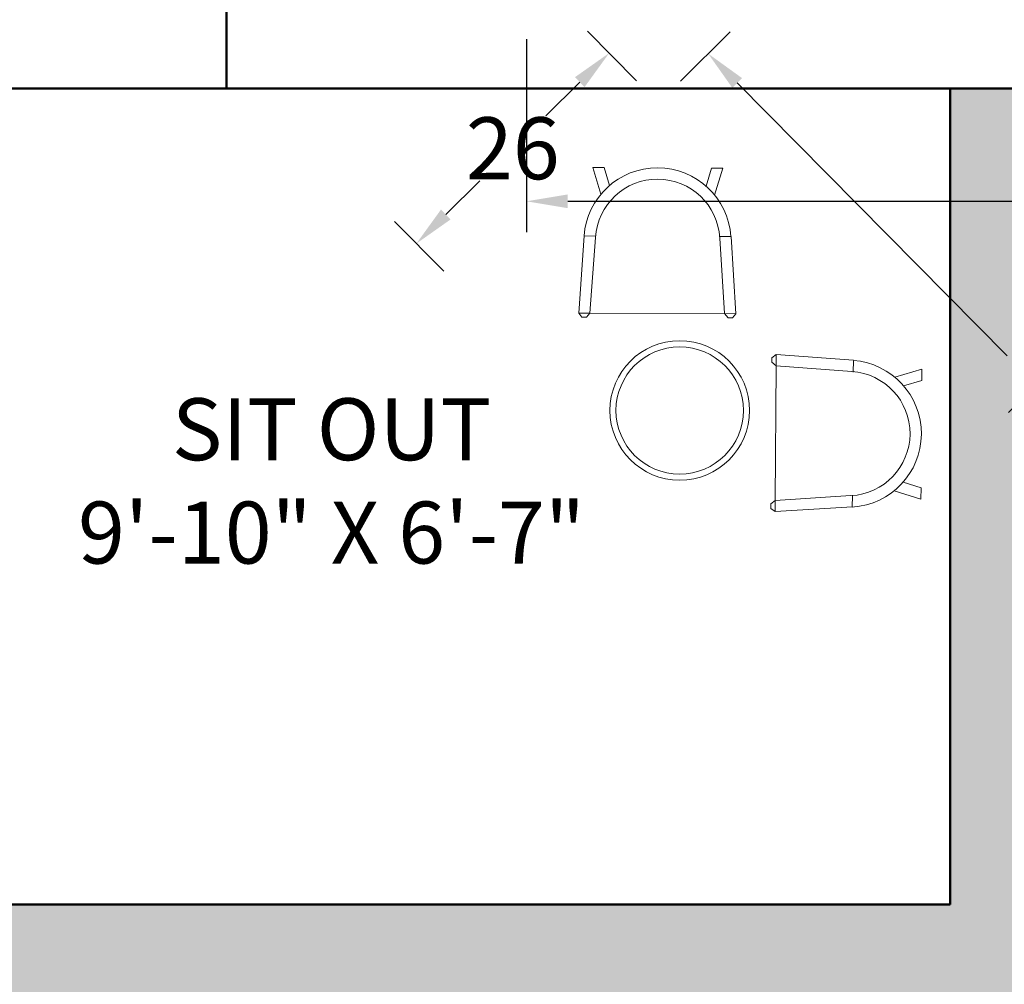
# Model space of a CAD drawing. Units: inches. Extents: x -466983 to 1020, y 324 to 318697.
# Tile 10 of 97: x 641 to 736, y 417 to 511. Entities that reach past the tile are written whole.
import ezdxf

# ---------------------------------------------------------------- set-up
doc = ezdxf.new("R2010")
doc.units = ezdxf.units.IN
doc.header["$MEASUREMENT"] = 0
for name, color, linetype, lineweight in [('A-ANNO-DIMS', 2, 'Continuous', 18), ('A-AREA-IDEN', 7, 'Continuous', 25), ('A-DOOR', 3, 'Continuous', 25), ('A-FLOR-PATT', 252, 'Continuous', 13), ('A-FURN', 8, 'Continuous', 18), ('A-WALL', 7, 'Continuous', 50)]:
    doc.layers.add(name, color=color, linetype=linetype, lineweight=lineweight)
doc.styles.get("Standard").update_dxf_attribs({"font": 'arial.ttf'})
doc.dimstyles.get("Standard").update_dxf_attribs({"dimtxt": 6, "dimasz": 4, "dimexe": 3, "dimexo": 3, "dimgap": 0.09, "dimtad": 0, "dimtih": 1, "dimtoh": 1, "dimdec": 1, "dimzin": 0, "dimdsep": 46, "dimlunit": 3, "dimtxsty": 'Standard', "dimcen": 0.09, "dimadec": 0, "dimazin": 0, "dimtfac": 1, "dimtdec": 1, "dimtofl": 0, "dimtmove": 0, "dimatfit": 3, "dimfxl": 1, "dimtolj": 1, "dimtzin": 0, "dimarcsym": 0})

# ---------------------------------------------------------------- blocks, each defined once
blk = doc.blocks.new('*U41')
for p, q in [((0, 0), (0, -6)), ((40, 0), (40, -6))]:
    blk.add_line(p, q)
blk.add_lwpolyline([(0, 0), (0, 40), (1.75, 40), (1.75, 0)], close=True)
blk.add_arc((0, 0), 40, 0, 90)
blk = doc.blocks.new('Chairs With Tea Table')
for p, q in [((2478.49, 1032.25), (2476.67, 1030.43)), ((2478.49, 1032.25), (2481.53, 1026.6)), ((2542.64, 1032.25), (2539.6, 1026.6)), ((2542.64, 1032.25), (2544.46, 1030.43)), ((2476.67, 1030.43), (2478.7, 1026.65)), ((2544.46, 1030.43), (2542.43, 1026.65)), ((2502.25, 1009.3), (2489.26, 1020.56)), ((2504.05, 1011.1), (2490.83, 1022.62)), ((2517.08, 1011.1), (2530.3, 1022.62)), ((2518.88, 1009.3), (2531.87, 1020.56)), ((2457.66, 1011.37), (2459.48, 1013.2)), ((2459.48, 1013.2), (2463.22, 1011.2)), ((2561.65, 1013.2), (2557.91, 1011.2)), ((2563.47, 1011.37), (2561.65, 1013.2)), ((2457.66, 1011.37), (2463.25, 1008.38)), ((2563.47, 1011.37), (2557.88, 1008.38)), ((2480.67, 987.66), (2502.25, 1009.3)), ((2540.46, 987.66), (2518.88, 1009.3)), ((2469.38, 1000.63), (2480.67, 987.66)), ((2551.75, 1000.63), (2540.46, 987.66)), ((2467.32, 999.05), (2478.9, 985.89)), ((2553.81, 999.05), (2542.23, 985.89))]:
    blk.add_line(p, q)
for points in [[(2488.94, 1020.72), (2490.81, 1022.59, 0.934026), (2467.3, 999.02), (2469.17, 1000.89)], [(2532.19, 1020.72), (2530.32, 1022.59, -0.934026), (2553.83, 999.02), (2551.96, 1000.89)]]:
    blk.add_lwpolyline(points, format="xyb")
for points in [[(2504.05, 1011.1), (2502.25, 1009.3), (2503.49, 1009.16), (2504.22, 1009.9)], [(2517.08, 1011.1), (2518.88, 1009.3), (2517.64, 1009.16), (2516.91, 1009.9)], [(2478.87, 985.86), (2480.67, 987.66), (2480.81, 986.43), (2480.08, 985.69)], [(2542.26, 985.86), (2540.46, 987.66), (2540.32, 986.43), (2541.05, 985.69)]]:
    blk.add_lwpolyline(points, close=True)
for radius in [15.83, 14.45]:
    blk.add_circle((2510.71, 986.6), radius)
for centre, start, end in [((2479.88, 1010.03), 48.307, 221.8389), ((2541.25, 1010.03), 318.1611, 131.693)]:
    blk.add_arc(centre, 14.1, start, end)
blk = doc.blocks.new('*D70')
at = {"layer": 'A-ANNO-DIMS', "color": 0, "lineweight": -2, "transparency": 16777216}
for p, q in [((689.806, 508.686), (689.806, 490.005)), ((810.968, 508.686), (810.968, 490.005)), ((693.806, 493.005), (744.53, 493.005)), ((806.968, 493.005), (756.244, 493.005))]:
    blk.add_line(p, q, dxfattribs=at)
at = {"layer": 'A-ANNO-DIMS', "color": 0, "transparency": 16777216}
for points in [[(693.806, 493.671), (693.806, 492.338), (689.806, 493.005)], [(806.968, 493.671), (806.968, 492.338), (810.968, 493.005)]]:
    blk.add_solid(points, dxfattribs=at)
at = {"layer": 'Defpoints', "color": 0, "transparency": 16777216}
for p in [(689.806, 511.686), (810.968, 511.686), (810.968, 493.005)]:
    blk.add_point(p, dxfattribs=at)
at = {"layer": 'A-ANNO-DIMS', "color": 0, "transparency": 16777216, "insert": (750.387, 493.005), "char_height": 6, "attachment_point": 5}
blk.add_mtext('\\A1;121', dxfattribs=at)
blk = doc.blocks.new('*D113')
at = {"layer": 'A-ANNO-DIMS', "color": 0, "lineweight": -2, "transparency": 16777216}
for p, q in [((704.71, 504.652), (709.525, 509.413)), ((710.204, 504.46), (736.319, 478.049)), ((736.45, 472.553), (741.265, 477.314)), ((739.132, 475.204), (741.944, 472.36)), ((741.944, 472.36), (745.944, 472.36))]:
    blk.add_line(p, q, dxfattribs=at)
at = {"layer": 'A-ANNO-DIMS', "color": 0, "transparency": 16777216}
for points in [[(710.678, 504.928), (709.73, 503.991), (707.392, 507.304)], [(736.794, 478.517), (735.845, 477.58), (739.132, 475.204)]]:
    blk.add_solid(points, dxfattribs=at)
at = {"layer": 'Defpoints', "color": 0, "transparency": 16777216}
for p in [(702.577, 502.543), (739.132, 475.204), (734.317, 470.443)]:
    blk.add_point(p, dxfattribs=at)
at = {"layer": 'A-ANNO-DIMS', "color": 0, "transparency": 16777216, "insert": (783.502, 472.36), "char_height": 6, "attachment_point": 5}
blk.add_mtext('\\A1;TEA TABLE SET 45', dxfattribs=at)
blk = doc.blocks.new('*D114')
at = {"layer": 'A-ANNO-DIMS', "color": 0, "lineweight": -2, "transparency": 16777216}
for p, q in [((700.467, 504.676), (695.706, 509.491)), ((694.971, 504.545), (691.68, 501.29)), ((682.01, 491.729), (685.301, 494.984)), ((681.817, 486.234), (677.056, 491.049))]:
    blk.add_line(p, q, dxfattribs=at)
at = {"layer": 'A-ANNO-DIMS', "color": 0, "transparency": 16777216}
for points in [[(694.503, 505.019), (695.44, 504.071), (697.816, 507.358)], [(681.541, 492.203), (682.478, 491.255), (679.165, 488.916)]]:
    blk.add_solid(points, dxfattribs=at)
at = {"layer": 'Defpoints', "color": 0, "transparency": 16777216}
for p in [(697.816, 507.358), (702.577, 502.543), (683.926, 484.101)]:
    blk.add_point(p, dxfattribs=at)
at = {"layer": 'A-ANNO-DIMS', "color": 0, "transparency": 16777216, "insert": (688.49, 498.137), "char_height": 6, "attachment_point": 5}
blk.add_mtext('\\A1;26', dxfattribs=at)

msp = doc.modelspace()

# ---------------------------------------------------------------- hatches: boundary and pattern name
at = {"layer": 'A-FLOR-PATT', "transparency": 33554661}
h = msp.add_hatch(color=256, dxfattribs=at)
h.dxf.hatch_style = 1
h.set_gradient(color1=(19, 155, 72), color2=(0, 107, 0), name='CYLINDER')
h.paths.add_polyline_path([(813.806, 503.938), (730.806, 503.938), (730.806, 424.938), (612.806, 424.938), (612.806, 415.938), (442.806, 415.938), (442.806, 368.938), (813.806, 368.938)])
h.paths.add_polyline_path([(771.796, 407.07), (783.796, 407.07), (783.796, 371.07), (771.796, 371.07)], flags=16)
h.paths.add_polyline_path([(755.796, 407.07), (755.796, 371.07), (743.796, 371.07), (743.796, 407.07)], flags=16)
h.paths.add_polyline_path([(769.796, 404.07), (769.796, 374.07), (757.796, 374.07), (757.796, 404.07)], flags=16)
h.paths.add_polyline_path([(785.796, 404.07), (797.796, 404.07), (797.796, 374.07), (785.796, 374.07)], flags=16)
h.paths.add_polyline_path([(741.796, 404.07), (741.796, 374.07), (729.796, 374.07), (729.796, 404.07)], flags=16)
h.paths.add_polyline_path([(799.796, 407.07), (811.796, 407.07), (811.796, 371.07), (799.796, 371.07)], flags=16)
h.paths.add_polyline_path([(727.796, 407.07), (727.796, 371.07), (715.796, 371.07), (715.796, 407.07)], flags=16)
h.paths.add_polyline_path([(713.796, 404.07), (713.796, 374.07), (701.796, 374.07), (701.796, 404.07)], flags=16)
h.paths.add_polyline_path([(699.796, 407.07), (699.796, 371.07), (687.796, 371.07), (687.796, 407.07)], flags=16)
h.paths.add_polyline_path([(685.796, 404.07), (685.796, 374.07), (673.796, 374.07), (673.796, 404.07)], flags=16)
h.paths.add_polyline_path([(671.796, 407.07), (671.796, 371.07), (659.796, 371.07), (659.796, 407.07)], flags=16)
h.paths.add_polyline_path([(657.796, 404.07), (657.796, 374.07), (645.796, 374.07), (645.796, 404.07)], flags=16)
h.paths.add_polyline_path([(643.796, 407.07), (643.796, 371.07), (631.796, 371.07), (631.796, 407.07)], flags=16)
h.paths.add_polyline_path([(629.796, 404.07), (629.796, 374.07), (617.796, 374.07), (617.796, 404.07)], flags=16)
h.paths.add_polyline_path([(615.796, 407.07), (615.796, 371.07), (603.796, 371.07), (603.796, 407.07)], flags=16)
h.paths.add_polyline_path([(601.796, 404.07), (601.796, 374.07), (589.796, 374.07), (589.796, 404.07)], flags=16)
at = {"layer": 'A-FLOR-PATT'}
h = msp.add_hatch(dxfattribs=at)
h.set_pattern_fill('GRASS', color=256, scale=6)
h.set_pattern_definition([(90, (-1212.4137, -290.035), (-4.242641, 4.242641), [1.125, -7.360281]), (45, (-1212.4137, -290.035), (-4.24264, 4.24264), [1.125, -4.875]), (135, (-1212.4137, -290.035), (-4.24264, -4.24264), [1.125, -4.875])])
h.paths.add_polyline_path([(813.806, 503.938), (730.806, 503.938), (730.806, 424.938), (612.806, 424.938), (612.806, 415.938), (442.806, 415.938), (442.806, 368.938), (813.806, 368.938)])
h.paths.add_polyline_path([(589.796, 404.07), (601.796, 404.07), (601.796, 374.07), (589.796, 374.07)], flags=16)
h.paths.add_polyline_path([(603.796, 407.07), (615.796, 407.07), (615.796, 371.07), (603.796, 371.07)], flags=16)
h.paths.add_polyline_path([(617.796, 404.07), (629.796, 404.07), (629.796, 374.07), (617.796, 374.07)], flags=16)
h.paths.add_polyline_path([(631.796, 407.07), (643.796, 407.07), (643.796, 371.07), (631.796, 371.07)], flags=16)
h.paths.add_polyline_path([(645.796, 404.07), (657.796, 404.07), (657.796, 374.07), (645.796, 374.07)], flags=16)
h.paths.add_polyline_path([(659.796, 407.07), (671.796, 407.07), (671.796, 371.07), (659.796, 371.07)], flags=16)
h.paths.add_polyline_path([(673.796, 404.07), (685.796, 404.07), (685.796, 374.07), (673.796, 374.07)], flags=16)
h.paths.add_polyline_path([(687.796, 407.07), (699.796, 407.07), (699.796, 371.07), (687.796, 371.07)], flags=16)
h.paths.add_polyline_path([(701.796, 404.07), (713.796, 404.07), (713.796, 374.07), (701.796, 374.07)], flags=16)
h.paths.add_polyline_path([(715.796, 407.07), (727.796, 407.07), (727.796, 371.07), (715.796, 371.07)], flags=16)
h.paths.add_polyline_path([(729.796, 404.07), (741.796, 404.07), (741.796, 374.07), (729.796, 374.07)], flags=16)
h.paths.add_polyline_path([(743.796, 407.07), (755.796, 407.07), (755.796, 371.07), (743.796, 371.07)], flags=16)
h.paths.add_polyline_path([(757.796, 404.07), (769.796, 404.07), (769.796, 374.07), (757.796, 374.07)], flags=16)
h.paths.add_polyline_path([(771.796, 407.07), (783.796, 407.07), (783.796, 371.07), (771.796, 371.07)], flags=16)
h.paths.add_polyline_path([(785.796, 404.07), (797.796, 404.07), (797.796, 374.07), (785.796, 374.07)], flags=16)
h.paths.add_polyline_path([(799.796, 407.07), (811.796, 407.07), (811.796, 371.07), (799.796, 371.07)], flags=16)

# ---------------------------------------------------------------- linework, layer by layer
at = {"layer": 'A-WALL'}
for p, q in [((660.806, 503.938), (660.806, 512.938)), ((813.806, 503.938), (618.806, 503.938)), ((730.806, 503.938), (730.806, 424.938)), ((730.806, 424.938), (612.806, 424.938))]:
    msp.add_line(p, q, dxfattribs=at)

# ---------------------------------------------------------------- block references
at = {"layer": 'A-DOOR', "xscale": 1.05, "yscale": 1.05, "zscale": 1.05}
msp.add_blockref('*U41', (618.806, 510.238), dxfattribs=at)
at = {"layer": 'A-FURN', "xscale": 0.426612482737599, "yscale": 0.426612482737599, "zscale": 0.426612482737599, "rotation": 314.6774666770456}
msp.add_blockref('Chairs With Tea Table', (-347.755, 938.45), dxfattribs=at)

# ---------------------------------------------------------------- texts
at = {"layer": 'A-AREA-IDEN', "insert": (556.173, 473.937), "char_height": 6, "attachment_point": 1}
msp.add_mtext_dynamic_manual_height_columns('\\pxqc;{\\fArial|b1|i0|c0|p34;SIT OUT\\P9\'-10" X 6\'-7"}', width=229.55829, gutter_width=1, heights=[0], dxfattribs=at)

# ---------------------------------------------------------------- dimensions: what is measured, and where the dimension line sits
at = {"layer": 'A-ANNO-DIMS'}
dim = msp.add_linear_dim(base=(810.968, 493.005), p1=(689.806, 511.686), p2=(810.968, 511.686), dimstyle='Standard', override={"dimdec": 0, "dimlfac": 1, "dimrnd": 0, "dimzin": 0, "dimdsep": 46, "dimlunit": 2}, dxfattribs=at)
dim.commit()
dim.dimension.update_dxf_attribs({"geometry": '*D70', "text_midpoint": (750.387, 493.005)})
dim = msp.add_linear_dim(base=(697.816, 507.358), p1=(683.926, 484.101), p2=(702.577, 502.543), angle=44.67747, dimstyle='Standard', override={"dimdec": 0, "dimlfac": 1, "dimrnd": 0, "dimzin": 0, "dimdsep": 46, "dimlunit": 2}, dxfattribs=at)
dim.commit()
dim.dimension.update_dxf_attribs({"geometry": '*D114', "text_midpoint": (688.49, 498.137)})
dim = msp.add_linear_dim(base=(739.132, 475.204), p1=(702.577, 502.543), p2=(734.317, 470.443), angle=314.67747, text='TEA TABLE SET <>', dimstyle='Standard', override={"dimdec": 0, "dimlfac": 1, "dimrnd": 0, "dimzin": 0, "dimdsep": 46, "dimlunit": 2}, dxfattribs=at)
dim.commit()
dim.dimension.update_dxf_attribs({"geometry": '*D113', "text_midpoint": (783.502, 472.36)})

doc.saveas('drawing.dxf')
